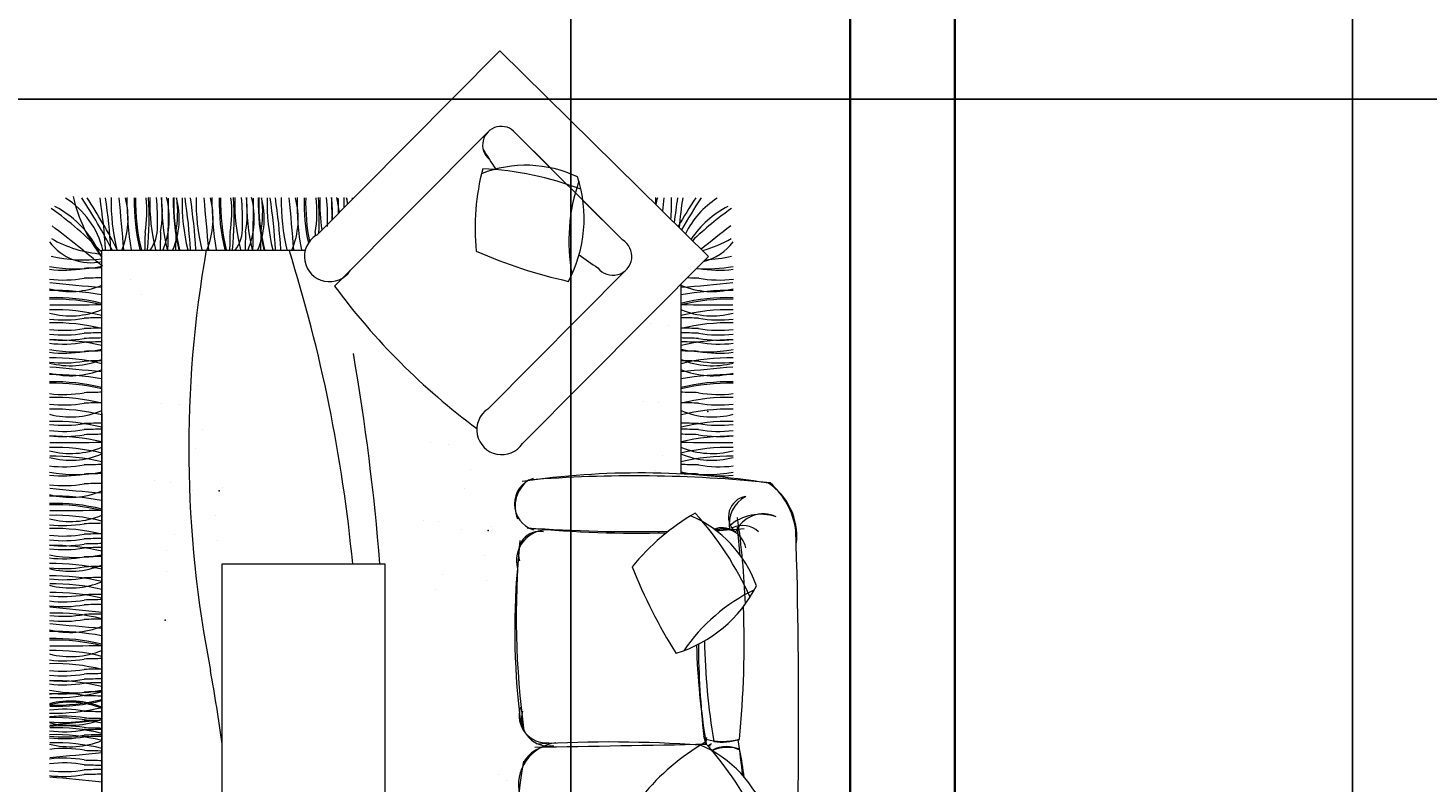
# Model space of a CAD drawing. Units: inches. Extents: x 502 to 1235, y -850 to 110.
# Tile 7 of 9: x 931 to 1051, y -277 to -212. Entities that reach past the tile are written whole.
import ezdxf

# ---------------------------------------------------------------- set-up
doc = ezdxf.new("R2010")
doc.units = ezdxf.units.IN
doc.header["$MEASUREMENT"] = 0
doc.layers.add('A-ANNO-DIMS', color=2, linetype='Continuous', lineweight=18)
doc.layers.add('WALL', color=1, linetype='Continuous', lineweight=35)
doc.layers.add('furniture', color=50, linetype='Continuous', lineweight=13, transparency=0.8)
doc.styles.get("Standard").update_dxf_attribs({"font": 'arial.ttf'})
doc.dimstyles.get("Standard").update_dxf_attribs({"dimtxt": 0.18, "dimasz": 0.18, "dimexe": 0.18, "dimexo": 0.0625, "dimgap": 0.09, "dimtad": 0, "dimtih": 1, "dimtoh": 1, "dimdec": 1, "dimzin": 0, "dimdsep": 46, "dimlunit": 4, "dimtxsty": 'Standard', "dimcen": 0.09, "dimadec": 0, "dimazin": 0, "dimtfac": 1, "dimtdec": 1, "dimtofl": 0, "dimtmove": 0, "dimatfit": 3, "dimfxl": 1, "dimtolj": 1, "dimtzin": 0, "dimarcsym": 0})

# ---------------------------------------------------------------- blocks, each defined once
blk = doc.blocks.new('_ArchTick')
at = {"color": 0, "linetype": 'ByBlock', "const_width": 0.15}
blk.add_lwpolyline([(-0.5, -0.5), (0.5, 0.5)], dxfattribs=at)
blk = doc.blocks.new('*D7')
at = {"layer": 'A-ANNO-DIMS', "color": 0, "lineweight": -2, "transparency": 16777216}
for p, q in [((1043.54, -60.85), (1044.72, -60.85)), ((1044.54, -60.85), (1044.54, -551.48)), ((1043.54, -551.48), (1044.72, -551.48))]:
    blk.add_line(p, q, dxfattribs=at)
at = {"layer": 'Defpoints', "color": 0, "transparency": 16777216}
for p in [(1010.39, -60.85), (1010.39, -551.48), (1044.54, -551.48)]:
    blk.add_point(p, dxfattribs=at)
at = {"layer": 'A-ANNO-DIMS', "color": 0, "lineweight": -2, "transparency": 16777216, "xscale": 5, "yscale": 5, "zscale": 5}
for p, rotation in [((1044.54, -60.85), 90), ((1044.54, -551.48), 270)]:
    blk.add_blockref('_ArchTick', p, dxfattribs=dict(at, rotation=rotation))
at = {"layer": 'A-ANNO-DIMS', "color": 0, "transparency": 16777216, "insert": (1036.52, -306.16), "char_height": 8, "attachment_point": 5, "rotation": 90}
blk.add_mtext("\\A1;42'", dxfattribs=at)
blk = doc.blocks.new('*D28')
at = {"layer": 'A-ANNO-DIMS', "color": 0, "lineweight": -2, "transparency": 16777216}
for p, q in [((770.85, -217.85), (1235.01, -217.85)), ((1234.83, -218.03), (1234.83, -255.91)), ((1234.83, -294.17), (1234.83, -256.28)), ((770.85, -294.35), (1235.01, -294.35))]:
    blk.add_line(p, q, dxfattribs=at)
at = {"layer": 'A-ANNO-DIMS', "color": 0, "transparency": 16777216}
for points in [[(1234.8, -218.03), (1234.86, -218.03), (1234.83, -217.85)], [(1234.8, -294.17), (1234.86, -294.17), (1234.83, -294.35)]]:
    blk.add_solid(points, dxfattribs=at)
at = {"layer": 'Defpoints', "color": 0, "transparency": 16777216}
for p in [(770.79, -217.85), (770.79, -294.35), (1234.83, -294.35)]:
    blk.add_point(p, dxfattribs=at)
at = {"layer": 'A-ANNO-DIMS', "color": 0, "transparency": 16777216, "insert": (1234.83, -256.1), "char_height": 0.18, "attachment_point": 5}
blk.add_mtext('\\A1;6\'-4 1/2"', dxfattribs=at)
blk = doc.blocks.new('*D29')
at = {"layer": 'A-ANNO-DIMS', "color": 0, "lineweight": -2, "transparency": 16777216}
for p, q in [((644.45, -193.85), (1235.01, -193.85)), ((1234.83, -194.03), (1234.83, -205.66)), ((1234.83, -217.67), (1234.83, -206.03)), ((644.45, -217.85), (1235.01, -217.85))]:
    blk.add_line(p, q, dxfattribs=at)
at = {"layer": 'A-ANNO-DIMS', "color": 0, "transparency": 16777216}
for points in [[(1234.8, -194.03), (1234.86, -194.03), (1234.83, -193.85)], [(1234.8, -217.67), (1234.86, -217.67), (1234.83, -217.85)]]:
    blk.add_solid(points, dxfattribs=at)
at = {"layer": 'Defpoints', "color": 0, "transparency": 16777216}
for p in [(644.39, -193.85), (644.39, -217.85), (1234.83, -217.85)]:
    blk.add_point(p, dxfattribs=at)
at = {"layer": 'A-ANNO-DIMS', "color": 0, "transparency": 16777216, "insert": (1234.83, -205.85), "char_height": 0.18, "attachment_point": 5}
blk.add_mtext('\\A1;2\'-0"', dxfattribs=at)
blk = doc.blocks.new('*D43')
at = {"layer": 'A-ANNO-DIMS', "color": 0, "lineweight": -2, "transparency": 16777216}
for p, q in [((977.39, -422.28), (977.39, 63.98)), ((977.57, 63.8), (989.06, 63.8)), ((1001.21, 63.8), (989.72, 63.8)), ((1001.39, -422.28), (1001.39, 63.98))]:
    blk.add_line(p, q, dxfattribs=at)
at = {"layer": 'A-ANNO-DIMS', "color": 0, "transparency": 16777216}
for points in [[(977.57, 63.83), (977.57, 63.77), (977.39, 63.8)], [(1001.21, 63.83), (1001.21, 63.77), (1001.39, 63.8)]]:
    blk.add_solid(points, dxfattribs=at)
at = {"layer": 'Defpoints', "color": 0, "transparency": 16777216}
for p in [(1001.39, 63.8), (977.39, -422.35), (1001.39, -422.35)]:
    blk.add_point(p, dxfattribs=at)
at = {"layer": 'A-ANNO-DIMS', "color": 0, "transparency": 16777216, "insert": (989.39, 63.8), "char_height": 0.18, "attachment_point": 5}
blk.add_mtext('\\A1;2\'-0"', dxfattribs=at)

msp = doc.modelspace()

# ---------------------------------------------------------------- linework, layer by layer
at = {"layer": 'furniture'}
for p, q in [((971.31, -213.69), (955.54, -229.55)), ((989.22, -231.37), (971.31, -213.69)), ((957.1, -233.92), (970.29, -220.66)), ((981.84, -229.94), (972.65, -220.76)), ((975.64, -223.75), (972.65, -220.76)), ((981.84, -229.94), (978.44, -226.55)), ((943.79, -227.99), (943.79, -227.99)), ((943.83, -228.42), (943.83, -228.42)), ((951.09, -227.99), (951.09, -227.99)), ((951.13, -228.42), (951.13, -228.42)), ((937.11, -319.68), (937.11, -230.81)), ((937.11, -230.81), (954.59, -230.81)), ((989.22, -231.37), (973.24, -247.44)), ((935.71, -232.22), (935.71, -232.22)), ((935.71, -232.22), (935.71, -232.22)), ((935.71, -232.22), (935.71, -232.22)), ((935.97, -233.3), (935.97, -233.3)), ((935.97, -233.3), (935.97, -233.3)), ((935.97, -233.3), (935.97, -233.3)), ((982.16, -232.5), (970.27, -244.47)), ((988, -233.3), (988, -233.3)), ((988, -233.3), (988, -233.3)), ((988, -233.3), (988, -233.3)), ((988.26, -232.22), (988.26, -232.22)), ((988.26, -232.22), (988.26, -232.22)), ((988.26, -232.22), (988.26, -232.22)), ((939.54, -233.32), (939.54, -233.32)), ((986.86, -233.74), (986.86, -250.05)), ((940.49, -234.66), (940.49, -234.66)), ((987.32, -235.64), (987.32, -235.64)), ((987.32, -235.64), (987.32, -235.64)), ((984.23, -237.14), (984.23, -237.14)), ((985.8, -237.26), (985.8, -237.26)), ((987.7, -239.45), (987.7, -239.45)), ((987.15, -241.03), (987.15, -241.03)), ((945.34, -242.46), (945.34, -242.46)), ((945.34, -242.46), (945.34, -242.46)), ((942.24, -243.96), (942.24, -243.96)), ((943.82, -244.08), (943.82, -244.08)), ((983.6, -243.83), (983.6, -243.83)), ((984.95, -243.93), (984.95, -243.93)), ((937.11, -244.85), (937.11, -319.68)), ((986.89, -244.62), (986.89, -244.62)), ((989.49, -244.36), (989.49, -244.36)), ((945.72, -246.27), (945.72, -246.27)), ((968.43, -245.87), (968.43, -245.87)), ((968.43, -245.87), (968.43, -245.87)), ((965.33, -247.37), (965.33, -247.37)), ((966.91, -247.49), (966.91, -247.49)), ((988.85, -246.83), (988.85, -246.83)), ((945.16, -247.85), (945.16, -247.85)), ((985.3, -248.45), (985.3, -248.45)), ((968.81, -249.68), (968.81, -249.68)), ((984.66, -249.78), (984.66, -249.78)), ((989.03, -248.94), (989.03, -248.94)), ((941.62, -250.65), (941.62, -250.65)), ((942.97, -250.75), (942.97, -250.75)), ((947.51, -251.18), (947.51, -251.18)), ((968.25, -251.26), (968.25, -251.26)), ((944.9, -251.44), (944.9, -251.44)), ((946.87, -253.65), (946.87, -253.65)), ((964.71, -254.06), (964.71, -254.06)), ((966.06, -254.16), (966.06, -254.16)), ((967.99, -254.85), (967.99, -254.85)), ((970.6, -254.59), (970.6, -254.59)), ((943.32, -255.27), (943.32, -255.27)), ((947.05, -255.76), (947.05, -255.76)), ((942.68, -256.6), (942.68, -256.6)), ((969.96, -257.06), (969.96, -257.06)), ((942.64, -258.44), (942.64, -258.44)), ((947.46, -257.76), (961.43, -257.76)), ((947.46, -291.3), (947.46, -257.76)), ((961.43, -257.76), (961.43, -291.3)), ((966.41, -258.68), (966.41, -258.68)), ((970.14, -259.17), (970.14, -259.17)), ((965.77, -260.01), (965.77, -260.01)), ((935.71, -268.94), (935.71, -268.94)), ((935.71, -269.04), (935.71, -269.04)), ((935.71, -272.07), (935.71, -272.07)), ((971.18, -275.86), (971.18, -275.86)), ((971.18, -275.86), (971.18, -275.86)), ((971.91, -276.35), (971.91, -276.35)), ((971.91, -276.35), (971.91, -276.35))]:
    msp.add_line(p, q, dxfattribs=at)
for centre, radius, start, end in [((971.42, -221.79), 1.6, 40.1092, 229.8908), ((996.78, -205.96), 31.42, 211.0867, 214.727), ((973.54, -233.83), 10.3, 64.4501, 111.7699), ((989.36, -228.95), 20.19, 165.3068, 185.5663), ((968.53, -251.07), 27.27, 69.0815, 87.2768), ((967, -228.09), 11.54, 332.0126, 17.9429), ((992.85, -230), 15.62, 160.9005, 190.6513), ((915.4, -251.75), 30.04, 43.716, 54.6847), ((929.13, -234.72), 8.61, 22.1181, 62.6967), ((930.08, -232.58), 7.35, 13.9935, 57.7288), ((947.54, -223.25), 13.24, 192.9523, 218.0769), ((893.44, -253.76), 50.12, 27.2669, 33.1781), ((893.89, -253.75), 50.12, 27.2669, 33.1781), ((888.83, -233.63), 48.68, 3.3644, 8.6229), ((889.29, -233.62), 48.68, 3.3644, 8.6229), ((954.94, -226.72), 17.03, 178.6331, 193.8573), ((740.82, -246.43), 198.79, 4.5146, 5.8017), ((932.39, -228.12), 6.98, 337.3098, 14.8613), ((961.88, -226.7), 22.61, 179.0195, 190.4039), ((956.92, -226.73), 17.03, 178.6331, 193.8573), ((957.04, -226.73), 17.03, 178.6331, 193.8573), ((930.87, -227.53), 10.11, 349.9349, 6.8829), ((918.17, -228.12), 23.01, 353.3702, 4.5064), ((958.26, -226.72), 17.03, 178.6331, 193.8573), ((926.14, -228.08), 15.76, 357.4435, 6.4413), ((932.2, -227.52), 10.11, 349.9349, 6.8829), ((959.27, -226.71), 17.03, 178.6331, 193.8573), ((935.93, -228.1), 6.98, 337.3098, 14.8613), ((797.03, -227.36), 145.8, 358.628, 0.3934), ((936.78, -228.11), 6.98, 337.3098, 14.8613), ((960.27, -226.73), 17.03, 178.6331, 193.8573), ((960.32, -226.72), 17.03, 178.6331, 193.8573), ((933.52, -227.53), 10.11, 349.9349, 6.8829), ((961.03, -226.73), 17.03, 178.6331, 193.8573), ((896.13, -233.63), 48.68, 3.3644, 8.6229), ((896.59, -233.62), 48.68, 3.3644, 8.6229), ((962.24, -226.72), 17.03, 178.6331, 193.8573), ((748.12, -246.43), 198.79, 4.5146, 5.8017), ((939.69, -228.12), 6.98, 337.3098, 14.8613), ((969.18, -226.7), 22.61, 179.0195, 190.4039), ((964.22, -226.73), 17.03, 178.6331, 193.8573), ((964.34, -226.73), 17.03, 178.6331, 193.8573), ((938.17, -227.53), 10.11, 349.9349, 6.8829), ((925.47, -228.12), 23.01, 353.3702, 4.5064), ((965.56, -226.72), 17.03, 178.6331, 193.8573), ((933.44, -228.08), 15.76, 357.4435, 6.4413), ((939.5, -227.52), 10.11, 349.9349, 6.8829), ((966.57, -226.71), 17.03, 178.6331, 193.8573), ((943.23, -228.1), 6.98, 337.3098, 14.8613), ((804.33, -227.36), 145.8, 358.628, 0.3934), ((944.08, -228.11), 6.98, 337.3098, 14.8613), ((967.57, -226.73), 17.03, 178.6331, 193.8573), ((967.62, -226.72), 17.03, 178.6331, 193.8573), ((940.82, -227.53), 10.11, 349.9349, 6.8829), ((968.33, -226.73), 17.03, 178.6331, 193.8573), ((903.44, -233.63), 48.68, 3.3644, 8.6229), ((903.89, -233.62), 48.68, 3.3644, 8.6229), ((969.55, -226.72), 17.03, 178.6331, 193.8573), ((755.43, -246.43), 198.79, 4.5146, 5.8017), ((947, -228.12), 6.98, 337.3098, 14.8613), ((976.49, -226.7), 22.61, 179.0195, 190.4039), ((971.52, -226.73), 17.03, 178.6331, 191.8302), ((971.65, -226.73), 17.03, 178.6331, 191.3519), ((945.48, -227.53), 10.11, 349.9349, 6.8829), ((932.78, -228.12), 23.01, 356.9677, 4.5064), ((972.87, -226.72), 17.03, 178.6331, 187.9798), ((940.75, -228.08), 15.76, 357.4435, 6.4413), ((973.87, -226.71), 17.03, 178.6331, 184.9238), ((946.81, -227.52), 10.11, 356.2453, 6.8829), ((950.54, -228.1), 6.98, 4.2757, 14.8613), ((811.63, -227.36), 145.8, 359.8849, 0.3934), ((974.93, -226.72), 17.03, 178.6331, 181.5238), ((951.39, -228.11), 6.98, 10.6592, 14.8613), ((948.13, -227.53), 10.11, 3.8173, 6.8829), ((975.64, -226.73), 17.03, 178.6331, 179.1046), ((962.09, -226.7), 22.61, 359.4753, 0.9805), ((991.58, -228.12), 6.98, 165.1387, 170.0752), ((1183.15, -246.43), 198.79, 174.1983, 174.5236), ((969.03, -226.72), 17.03, 355.0538, 1.3669), ((1034.69, -233.62), 48.68, 171.3771, 173.9203), ((1030.08, -253.75), 50.12, 146.8219, 150.1356), ((1035.14, -233.63), 48.68, 171.3771, 174.3888), ((1030.53, -253.76), 50.12, 146.8219, 150.5026), ((993.89, -232.58), 7.35, 122.2712, 154.6274), ((994.84, -234.72), 8.61, 117.3033, 145.7016), ((1008.57, -251.75), 30.04, 125.3153, 133.6457), ((848.78, -338.11), 137.94, 50.1568, 52.4559), ((1053.53, -232.86), 112.76, 178.1891, 178.9775), ((938.84, -228.95), 3.05, 321.6564, 3.1744), ((1054.86, -232.85), 112.76, 178.1891, 178.9775), ((1056.18, -232.86), 112.76, 178.1891, 178.9775), ((1060.83, -232.86), 112.76, 178.1891, 178.9775), ((946.15, -228.95), 3.05, 321.6564, 3.1744), ((1062.16, -232.85), 112.76, 178.1891, 178.9775), ((1063.48, -232.86), 112.76, 178.1891, 178.9775), ((956.66, -231.38), 2.15, 121.4693, 326.9076), ((1068.14, -232.86), 112.76, 178.1891, 178.3576), ((1075.19, -338.11), 137.94, 127.5441, 128.8901), ((936.15, -227.55), 4.35, 215.9057, 282.8054), ((937.87, -220.97), 10.21, 240.135, 265.7243), ((1042.34, -247.9), 97.76, 169.9275, 191.2246), ((828.12, -270.19), 131.13, 5.4421, 17.4799), ((981.01, -231.35), 1.63, 217.6748, 59.5181), ((986.1, -220.97), 10.21, 284.6792, 299.865), ((987.82, -227.55), 4.35, 282.9777, 324.0943), ((935.58, -219.38), 12.28, 256.7215, 277.1491), ((986.61, -191.34), 43.2, 246.3371, 257.4176), ((996.78, -205.96), 31.42, 233.5454, 237.1144), ((988.39, -219.38), 12.28, 272.5322, 283.2785), ((933.83, -222.43), 10.11, 263.1171, 280.0651), ((933.82, -223.28), 10.11, 263.1171, 280.0651), ((934.83, -221.11), 11.32, 258.7545, 281.5888), ((939.16, -345.09), 112.76, 91.0225, 91.8109), ((939.15, -345.94), 112.76, 91.0225, 91.8109), ((984.82, -345.94), 112.76, 88.1891, 88.6709), ((989.14, -221.11), 11.32, 265.1756, 281.2455), ((990.14, -222.43), 10.11, 259.9349, 276.8829), ((990.15, -223.28), 10.11, 259.9349, 276.8829), ((933.01, -256.9), 22.61, 79.5961, 90.9805), ((934.42, -227.4), 6.98, 255.1387, 292.6902), ((952.74, -35.84), 198.79, 264.1983, 265.4854), ((1004.81, -198.48), 59.43, 216.6049, 233.3387), ((989.55, -227.4), 6.98, 247.3098, 284.8613), ((971.23, -35.84), 198.79, 274.5146, 275.8017), ((990.96, -256.9), 22.61, 89.0195, 100.4039), ((933.03, -251.93), 17.03, 76.1427, 91.3669), ((933.03, -252.06), 17.03, 76.1427, 91.3669), ((933.66, -89.73), 145.8, 269.6066, 271.372), ((990.31, -89.73), 145.8, 268.628, 270.3934), ((990.94, -251.93), 17.03, 88.6331, 103.8573), ((990.94, -252.06), 17.03, 88.6331, 103.8573), ((933.03, -252.97), 17.03, 76.1427, 91.3669), ((933.83, -226.71), 10.11, 263.1171, 280.0651), ((934.42, -229.49), 6.98, 255.1387, 292.6902), ((939.16, -349.37), 112.76, 91.0225, 91.8109), ((984.81, -349.37), 112.76, 88.1891, 88.9775), ((989.55, -229.49), 6.98, 247.3098, 284.8613), ((990.94, -252.97), 17.03, 88.6331, 103.8573), ((990.14, -226.71), 10.11, 259.9349, 276.8829), ((933.03, -254.09), 17.03, 76.1427, 91.3669), ((933.83, -227.6), 10.11, 263.1171, 280.0651), ((933.83, -228), 10.11, 263.1171, 280.0651), ((939.16, -350.26), 112.76, 91.0225, 91.8109), ((939.16, -350.66), 112.76, 91.0225, 91.8109), ((984.81, -350.26), 112.76, 88.1891, 88.9775), ((984.81, -350.66), 112.76, 88.1891, 88.9775), ((990.94, -254.09), 17.03, 88.6331, 103.8573), ((990.14, -227.6), 10.11, 259.9349, 276.8829), ((990.14, -228), 10.11, 259.9349, 276.8829), ((933.83, -228.45), 10.11, 263.1171, 280.0651), ((933.02, -255.56), 17.03, 76.1427, 91.3669), ((933.83, -228.78), 10.11, 263.1171, 280.0651), ((939.16, -351.11), 112.76, 91.0225, 91.8109), ((939.16, -351.44), 112.76, 91.0225, 91.8109), ((984.81, -351.11), 112.76, 88.1891, 88.9775), ((984.81, -351.44), 112.76, 88.1891, 88.9775), ((990.95, -255.56), 17.03, 88.6331, 103.8573), ((990.14, -228.45), 10.11, 259.9349, 276.8829), ((990.14, -228.78), 10.11, 259.9349, 276.8829), ((933.83, -229.56), 10.11, 263.1171, 280.0651), ((933.02, -257.11), 17.03, 76.1427, 91.3669), ((933.82, -230.4), 10.11, 263.1171, 280.0651), ((934.83, -228.24), 11.32, 258.7545, 281.5888), ((934.41, -233.77), 6.98, 255.1387, 292.6902), ((939.16, -352.22), 112.76, 91.0225, 91.8109), ((939.15, -353.06), 112.76, 91.0225, 91.8109), ((758.48, -274.12), 203.18, 4.6196, 9.7513), ((984.81, -352.22), 112.76, 88.1891, 88.9775), ((984.82, -353.06), 112.76, 88.1891, 88.9775), ((989.14, -228.24), 11.32, 258.4112, 281.2455), ((990.95, -257.11), 17.03, 88.6331, 103.8573), ((989.56, -233.77), 6.98, 247.3098, 284.8613), ((990.14, -229.56), 10.11, 259.9349, 276.8829), ((990.15, -230.4), 10.11, 259.9349, 276.8829), ((933.01, -264.12), 22.61, 79.5961, 90.9805), ((934.42, -234.63), 6.98, 255.1387, 292.6902), ((952.74, -43.06), 198.79, 264.1983, 265.4854), ((989.55, -234.63), 6.98, 247.3098, 284.8613), ((971.23, -43.06), 198.79, 274.5146, 275.8017), ((990.96, -264.12), 22.61, 89.0195, 100.4039), ((933.03, -259.16), 17.03, 76.1427, 91.3669), ((933.03, -259.28), 17.03, 76.1427, 91.3669), ((990.94, -259.16), 17.03, 88.6331, 103.8573), ((990.94, -259.28), 17.03, 88.6331, 103.8573), ((933.83, -233.11), 10.11, 263.1171, 280.0651), ((933.03, -260.5), 17.03, 76.1427, 91.3669), ((933.83, -234.01), 10.11, 263.1171, 280.0651), ((939.16, -355.77), 112.76, 91.0225, 91.8109), ((939.16, -356.67), 112.76, 91.0225, 91.8109), ((984.81, -355.77), 112.76, 88.1891, 88.9775), ((984.81, -356.67), 112.76, 88.1891, 88.9775), ((990.94, -260.5), 17.03, 88.6331, 103.8573), ((990.14, -233.11), 10.11, 259.9349, 276.8829), ((990.14, -234.01), 10.11, 259.9349, 276.8829), ((933.02, -261.51), 17.03, 76.1427, 91.3669), ((934.41, -238.17), 6.98, 255.1387, 292.6902), ((971.46, -246.25), 2.14, 123.6335, 326.3665), ((990.95, -261.51), 17.03, 88.6331, 103.8573), ((989.56, -238.17), 6.98, 247.3098, 284.8613), ((933.02, -262.56), 17.03, 76.1427, 91.3669), ((933.83, -236.28), 10.11, 263.1171, 280.0651), ((933.84, -235.76), 10.11, 263.1171, 280.0651), ((939.16, -358.94), 112.76, 91.0225, 91.8109), ((939.17, -358.42), 112.76, 91.0225, 91.8109), ((984.8, -358.42), 112.76, 88.1891, 88.9775), ((984.81, -358.94), 112.76, 88.1891, 88.9775), ((990.95, -262.56), 17.03, 88.6331, 103.8573), ((990.13, -235.76), 10.11, 259.9349, 276.8829), ((990.14, -236.28), 10.11, 259.9349, 276.8829), ((933.83, -236.72), 10.11, 263.1171, 280.0651), ((933.02, -263.83), 17.03, 76.1427, 91.3669), ((933.66, -101.55), 145.8, 269.6066, 271.372), ((939.16, -359.38), 112.76, 91.0225, 91.8109), ((984.81, -359.38), 112.76, 88.1891, 88.9775), ((990.31, -101.55), 145.8, 268.628, 270.3934), ((990.95, -263.83), 17.03, 88.6331, 103.8573), ((990.14, -236.72), 10.11, 259.9349, 276.8829), ((933.03, -264.79), 17.03, 76.1427, 91.3669), ((934.42, -241.31), 6.98, 255.1387, 292.6902), ((934.42, -241.89), 6.98, 255.1387, 292.6902), ((933.04, -265.55), 17.03, 76.1427, 91.3669), ((989.55, -241.89), 6.98, 247.3098, 284.8613), ((990.93, -265.55), 17.03, 88.6331, 103.8573), ((989.55, -241.31), 6.98, 247.3098, 284.8613), ((990.94, -264.79), 17.03, 88.6331, 103.8573), ((933.83, -240.1), 10.11, 263.1171, 280.0651), ((933.83, -239.32), 10.11, 263.1171, 280.0651), ((934.83, -238.78), 11.32, 258.7545, 281.5888), ((939.16, -362.76), 112.76, 91.0225, 91.8109), ((939.16, -361.98), 112.76, 91.0225, 91.8109), ((983.31, -319.39), 69.43, 80.8079, 98.3514), ((984.81, -361.98), 112.76, 88.1891, 88.9775), ((984.81, -362.76), 112.76, 88.1891, 88.9775), ((989.14, -238.78), 11.32, 258.4112, 281.2455), ((990.14, -239.32), 10.11, 259.9349, 276.8829), ((990.14, -240.1), 10.11, 259.9349, 276.8829), ((933.82, -240.94), 10.11, 263.1171, 280.0651), ((952.74, -53.5), 198.79, 264.1983, 265.4854), ((939.15, -363.6), 112.76, 91.0225, 91.8109), ((974.86, -252.63), 2.31, 107.7157, 252.8428), ((975.39, -252.83), 2.78, 126.0678, 202.6723), ((982.86, -363.06), 112.85, 84.0627, 94.6253), ((991.35, -255.38), 5.46, 353.8792, 57.1093), ((990.12, -255.84), 6.68, 8.6549, 48.7104), ((933.01, -274.56), 22.61, 79.5961, 90.9805), ((934.42, -245.07), 6.98, 255.1387, 292.6902), ((992.7, -253.72), 1.76, 99.2916, 227.6289), ((993.67, -254.36), 2.68, 117.8433, 189.8684), ((933.03, -270.63), 17.03, 76.1427, 91.3669), ((933.03, -269.6), 17.03, 76.1427, 91.3669), ((933.03, -269.72), 17.03, 76.1427, 91.3669), ((934.42, -247.15), 6.98, 255.1387, 292.6902), ((933.66, -107.39), 145.8, 269.6066, 271.372), ((998.26, -270.84), 20.19, 120.3068, 140.5663), ((983.63, -263.1), 10.3, 19.4501, 66.7699), ((967.9, -271.76), 27.27, 24.0815, 42.2768), ((993.71, -257.62), 4.11, 71.2473, 131.1348), ((993.93, -256.08), 2.6, 64.8715, 156.7247), ((933.83, -244.37), 10.11, 263.1171, 280.0651), ((933.03, -271.76), 17.03, 76.1427, 91.3669), ((939.16, -367.03), 112.76, 91.0225, 91.8109), ((975.41, -257.52), 2.68, 87.6579, 194.0974), ((982.78, -130.25), 124.75, 265.8027, 271.3803), ((983.23, -152.49), 102.64, 264.7422, 271.3335), ((990.37, -256.43), 1.77, 57.7366, 112.2387), ((982.78, -130.25), 124.75, 273.1908, 273.7892), ((990.48, -256.75), 1.98, 10.6216, 109.193), ((983.23, -152.49), 102.64, 273.7101, 275.0653), ((992.14, -256.55), 2.07, 47.7203, 114.4461), ((922.4, -263.9), 70.05, 2.2017, 8.3067), ((907.86, -264.55), 84.43, 5.0871, 6.7491), ((497.35, -270.42), 499.62, 357.2697, 1.7875), ((933.83, -245.27), 10.11, 263.1171, 280.0651), ((933.83, -245.67), 10.11, 263.1171, 280.0651), ((933.83, -246.11), 10.11, 263.1171, 280.0651), ((939.16, -367.93), 112.76, 91.0225, 91.8109), ((939.16, -368.33), 112.76, 91.0225, 91.8109), ((939.16, -368.77), 112.76, 91.0225, 91.8109), ((1045.69, -262.34), 72.98, 174.8245, 187.7148), ((974.74, -256.84), 1.86, 80.2617, 201.0115), ((933.83, -247.22), 10.11, 263.1171, 280.0651), ((933.02, -273.22), 17.03, 76.1427, 91.3669), ((933.83, -246.44), 10.11, 263.1171, 280.0651), ((934.83, -245.9), 11.32, 258.7545, 281.5888), ((939.16, -369.88), 112.76, 91.0225, 91.8109), ((939.16, -369.1), 112.76, 91.0225, 91.8109), ((933.02, -274.77), 17.03, 76.1427, 91.3669), ((933.82, -248.07), 10.11, 263.1171, 280.0651), ((934.41, -251.43), 6.98, 255.1387, 292.6902), ((939.15, -370.73), 112.76, 91.0225, 91.8109), ((1034.38, -263.47), 61.8, 175.0781, 187.695), ((1022.91, -242.3), 43.2, 201.3371, 212.4176), ((933.02, -275.83), 17.03, 76.1427, 91.3669), ((933.84, -249.02), 10.11, 263.1171, 280.0651), ((934.42, -252.86), 6.98, 255.1387, 292.6902), ((933.04, -276.52), 17.03, 76.1427, 91.3669), ((939.17, -371.68), 112.76, 91.0225, 91.8109), ((983.06, -254.42), 11.54, 287.0126, 332.9429), ((933.04, -277.26), 17.03, 76.1427, 91.3669), ((933.84, -250.47), 10.11, 263.1171, 280.0651), ((933.84, -250.92), 10.11, 263.1171, 280.0651), ((939.17, -373.13), 112.76, 91.0225, 91.8109), ((939.17, -373.58), 112.76, 91.0225, 91.8109), ((999.99, -274.05), 15.62, 115.9005, 145.6513), ((933.82, -251.33), 10.11, 263.1171, 280.0651), ((933.04, -279.02), 17.03, 76.1427, 91.3669), ((897.72, -637.92), 378.04, 84.0165, 84.6992), ((933.85, -252.16), 10.11, 263.1171, 280.0651), ((939.15, -373.99), 112.76, 91.0225, 91.8109), ((939.18, -374.82), 112.76, 91.0225, 91.8109), ((907.86, -264.55), 84.43, 354.3639, 2.1219), ((933.84, -252.59), 10.11, 263.1171, 280.0651), ((934.42, -256.68), 6.98, 255.1387, 292.6902), ((952.74, -65.12), 198.79, 264.1983, 265.4854), ((939.17, -375.25), 112.76, 91.0225, 91.8109), ((933.01, -286.18), 22.61, 79.5961, 90.9805), ((933.03, -281.21), 17.03, 76.1427, 91.3669), ((933.03, -281.34), 17.03, 76.1427, 91.3669), ((1046.79, -263.37), 57.92, 181.0061, 189.6001), ((933.03, -282.25), 17.03, 76.1427, 91.3669), ((934.42, -258.76), 6.98, 255.1387, 292.6902), ((933.66, -119.01), 145.8, 269.6066, 271.372), ((1050.02, -262.98), 61.85, 181.6458, 189.5268), ((1066.11, -264.01), 77.76, 180.4949, 186.3291), ((933.83, -255.99), 10.11, 263.1171, 280.0651), ((933.03, -283.37), 17.03, 76.1427, 91.3669), ((933.83, -256.88), 10.11, 263.1171, 280.0651), ((939.16, -378.65), 112.76, 91.0225, 91.8109), ((939.16, -379.54), 112.76, 91.0225, 91.8109), ((759.42, -300.06), 189.94, 8.119, 10.0442), ((933.83, -257.28), 10.11, 263.1171, 280.0651), ((933.83, -257.73), 10.11, 263.1171, 280.0651), ((933.02, -284.84), 17.03, 76.1427, 91.3669), ((933.83, -258.05), 10.11, 263.1171, 280.0651), ((939.16, -379.94), 112.76, 91.0225, 91.8109), ((939.16, -380.39), 112.76, 91.0225, 91.8109), ((939.16, -380.72), 112.76, 91.0225, 91.8109), ((933.83, -258.83), 10.11, 263.1171, 280.0651), ((934.83, -257.52), 11.32, 258.7545, 281.5888), ((933.04, -252.23), 17.03, 268.6331, 283.8573), ((933.84, -279.02), 10.11, 79.9349, 96.8829), ((939.16, -381.49), 112.76, 91.0225, 91.8109), ((939.17, -156.36), 112.76, 268.1891, 268.9775), ((933.02, -253.57), 17.03, 268.6331, 283.8573), ((933.04, -252.88), 17.03, 268.6331, 283.8573), ((933.04, -252.98), 17.03, 268.6331, 283.8573), ((934.42, -276.53), 6.98, 67.3098, 104.8613), ((934.42, -276.63), 6.98, 67.3098, 104.8613), ((933.84, -280.37), 10.11, 79.9349, 96.8829), ((939.17, -157.71), 112.76, 268.1891, 268.9775), ((975.31, -270.8), 2.35, 162.9316, 275.1092), ((975.48, -271.09), 2.33, 163.4437, 271.8228), ((933.02, -288), 17.03, 76.1427, 91.3669), ((933.82, -261.29), 10.11, 263.1171, 280.0651), ((933.82, -281.79), 10.11, 79.9349, 96.8829), ((934.41, -264.66), 6.98, 255.1387, 292.6902), ((933.85, -280.96), 10.11, 79.9349, 96.8829), ((897.72, 104.8), 378.04, 275.3008, 275.9835), ((939.15, -383.95), 112.76, 91.0225, 91.8109), ((939.18, -158.3), 112.76, 268.1891, 268.9775), ((933.02, -289.47), 17.03, 76.1427, 91.3669), ((933.04, -288.87), 17.03, 76.1427, 91.3669), ((933.84, -262.08), 10.11, 263.1171, 280.0651), ((933.84, -262.53), 10.11, 263.1171, 280.0651), ((933.84, -262.67), 10.11, 263.1171, 280.0651), ((934.42, -266.5), 6.98, 255.1387, 292.6902), ((939.15, -159.13), 112.76, 268.1891, 268.9775), ((939.17, -384.74), 112.76, 91.0225, 91.8109), ((939.17, -385.19), 112.76, 91.0225, 91.8109), ((939.17, -385.33), 112.76, 91.0225, 91.8109), ((965.22, -280.01), 24.74, 15.9625, 17.4638), ((990.47, -267.25), 5.77, 254.0479, 284.2061), ((1108.91, -285.53), 120.55, 173.8872, 174.1215), ((990.38, -268.34), 4.74, 261.5362, 288.3493), ((927.74, -282.47), 64.75, 5.7795, 8.522), ((933.04, -290.16), 17.03, 76.1427, 91.3669), ((933.85, -283.74), 10.11, 79.9349, 96.8829), ((897.72, 102.02), 378.04, 275.3008, 275.9835), ((939.18, -161.08), 112.76, 268.1891, 268.9775), ((976.54, -276.76), 3.64, 96.5867, 193.4511), ((975.7, -276.08), 2.66, 84.9234, 155.6374), ((-20965.24, 1230594.14), 1231063.17, 271.02115817, 271.0218453), ((980.68, -381.02), 107.95, 85.8425, 93.2873), ((999.11, -290.54), 20.19, 120.3068, 140.5663), ((984.48, -282.8), 10.3, 19.4501, 66.7699), ((968.74, -291.45), 27.27, 24.0815, 42.2768), ((980.68, -381.02), 107.95, 85.3655, 85.4784), ((990.18, -274.51), 1.46, 119.1313, 132.0141), ((1059.84, -282.76), 70.83, 172.7245, 172.7726), ((990.73, -275.81), 2.34, 59.8319, 119.468), ((990.9, -276.97), 3.44, 73.3108, 112.6164), ((942.43, -282.94), 50.33, 7.803, 10.4557), ((933.82, -284.57), 10.11, 79.9349, 96.8829), ((933.84, -284.98), 10.11, 79.9349, 96.8829), ((939.15, -161.91), 112.76, 268.1891, 268.9775), ((939.17, -162.32), 112.76, 268.1891, 268.9775), ((1018.67, -282.68), 46.03, 170.0543, 190.4167), ((933.82, -265.92), 10.11, 263.1171, 280.0651), ((933.84, -265.51), 10.11, 263.1171, 280.0651), ((897.72, -652.51), 378.04, 84.0165, 84.6992), ((939.15, -388.58), 112.76, 91.0225, 91.8109), ((939.17, -388.17), 112.76, 91.0225, 91.8109)]:
    msp.add_arc(centre, radius, start, end, dxfattribs=at)
for p in [(989.18, -244.67), (947.2, -251.49), (970.29, -254.9), (942.55, -262.61)]:
    msp.add_point(p, dxfattribs=at)
at = {"layer": 'WALL'}
for p, q in [((1010.39, -615.85), (1010.39, -60.85)), ((1001.39, -418.35), (1001.39, -193.85))]:
    msp.add_line(p, q, dxfattribs=at)

# ---------------------------------------------------------------- dimensions: what is measured, and where the dimension line sits
at = {"layer": 'A-ANNO-DIMS'}
dim = msp.add_linear_dim(base=(1001.39, 63.8), p1=(977.39, -422.35), p2=(1001.39, -422.35), dimstyle='Standard', override={"dimdec": 1, "dimlfac": 1, "dimrnd": 0, "dimzin": 1, "dimdsep": 46, "dimlunit": 4, "dimfrac": 2}, dxfattribs=at)
dim.commit()
dim.dimension.update_dxf_attribs({"geometry": '*D43', "text_midpoint": (989.39, 63.8)})
dim = msp.add_linear_dim(base=(1044.54, -551.48), p1=(1010.39, -60.85), p2=(1010.39, -551.48), angle=90, text="42'", dimstyle='Standard', override={"dimtxt": 8, "dimasz": 5, "dimgap": 4, "dimtad": 1, "dimtih": 0, "dimblk1": 'ArchTick', "dimblk2": 'ArchTick', "dimsah": 1, "dimclrd": 0, "dimclre": 0, "dimclrt": 0, "dimfxlon": 1}, dxfattribs=at)
dim.commit()
dim.dimension.update_dxf_attribs({"geometry": '*D7', "text_midpoint": (1036.52, -306.16)})
for base, p1, p2, picture, middle in [((1234.83, -217.85), (644.39, -193.85), (644.39, -217.85), '*D29', (1234.83, -205.85)), ((1234.83, -294.35), (770.79, -217.85), (770.79, -294.35), '*D28', (1234.83, -256.1))]:
    dim = msp.add_linear_dim(base=base, p1=p1, p2=p2, angle=90, dimstyle='Standard', override={"dimdec": 1, "dimlfac": 1, "dimrnd": 0, "dimzin": 1, "dimdsep": 46, "dimlunit": 4, "dimfrac": 2}, dxfattribs=at)
    dim.commit()
    dim.dimension.update_dxf_attribs({"geometry": picture, "text_midpoint": middle})

doc.saveas('drawing.dxf')
